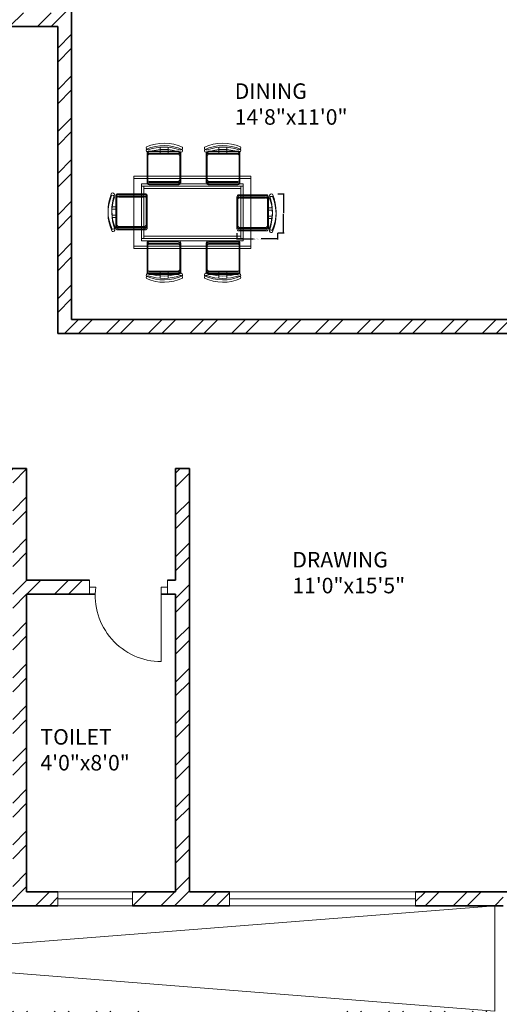
# Model space of a CAD drawing. Units: inches. Extents: x 1885 to 2748, y 783 to 2421.
# Tile 87 of 117: x 2294 to 2449, y 1850 to 2167. Entities that reach past the tile are written whole.
import ezdxf

# ---------------------------------------------------------------- set-up
doc = ezdxf.new("R2010")
doc.units = ezdxf.units.IN
for name, color, linetype, lineweight in [('A-ANNO-DIMS', 2, 'Continuous', 18), ('A-AREA-IDEN', 7, 'Continuous', 18), ('A-DOOR', 31, 'Continuous', 18), ('A-FLOR-OPEN', 8, 'Continuous', 13), ('A-FURN', 8, 'Continuous', 13), ('A-GLAZ', 181, 'Continuous', 18), ('A-WALL', 7, 'Continuous', 35)]:
    doc.layers.add(name, color=color, linetype=linetype, lineweight=lineweight)
doc.layers.add('A-WALL-PATT', color=85, linetype='Continuous', lineweight=13, true_color=0x58ba48)
doc.styles.get("Standard").update_dxf_attribs({"font": 'arial.ttf'})
doc.dimstyles.get("Standard").update_dxf_attribs({"dimtxt": 0.18, "dimasz": 0.18, "dimexe": 0.18, "dimexo": 0.0625, "dimgap": 0.09, "dimtad": 0, "dimtih": 1, "dimtoh": 1, "dimdec": 4, "dimzin": 0, "dimdsep": 46, "dimtxsty": 'Standard', "dimcen": 0.09, "dimadec": 0, "dimazin": 0, "dimtfac": 1, "dimtdec": 4, "dimtofl": 0, "dimtmove": 0, "dimatfit": 3, "dimfxl": 1, "dimtolj": 1, "dimtzin": 0, "dimarcsym": 0})

# ---------------------------------------------------------------- blocks, each defined once
blk = doc.blocks.new('WIN-60')
for p, q in [((0, 60), (4.5, 60)), ((0, 60), (0, 0)), ((4.5, 60), (2.25, 60)), ((2.25, 60), (2.25, 0)), ((4.5, 0), (4.5, 60)), ((2.25, 0), (0, 0)), ((0, 0), (4.5, 0))]:
    blk.add_line(p, q)
blk = doc.blocks.new('WIN-24')
for p, q in [((0, 4.5), (0, 0)), ((0, 4.5), (24, 4.5)), ((24, 2.25), (24, 4.5)), ((24, 4.5), (24, 0)), ((0, 0), (0, 2.25)), ((0, 2.25), (24, 2.25)), ((24, 0), (0, 0))]:
    blk.add_line(p, q)
blk = doc.blocks.new('TABLE-DINING-RECT')
for points in [[(0, 23.42), (37.78, 23.42), (37.78, 0.75), (0, 0.75)], [(0, 23.42), (37.78, 23.42), (37.78, 0.75), (0, 0.75)], [(0, 22.67), (37.78, 22.67), (37.78, 0), (0, 0)], [(0, 22.67), (37.78, 22.67), (37.78, 0), (0, 0)], [(2.51, 20.9), (35.26, 20.9), (35.26, 3.27), (2.51, 3.27)], [(2.51, 20.9), (35.26, 20.9), (35.26, 3.27), (2.51, 3.27)], [(2.51, 20.15), (35.26, 20.15), (35.26, 2.52), (2.51, 2.52)], [(2.51, 20.15), (35.26, 20.15), (35.26, 2.52), (2.51, 2.52)], [(3.27, 20.15), (34.5, 20.15), (34.5, 4.03), (3.27, 4.03)], [(3.27, 20.15), (34.5, 20.15), (34.5, 4.03), (3.27, 4.03)], [(3.27, 19.39), (34.5, 19.39), (34.5, 3.27), (3.27, 3.27)], [(3.27, 19.39), (34.5, 19.39), (34.5, 3.27), (3.27, 3.27)]]:
    blk.add_lwpolyline(points, close=True)
blk = doc.blocks.new('CHAIR-DINING-SIDE-B')
for points in [[(10.8, 3.27, 0.414214), (11.47, 3.94), (11.47, 12.73, 0.414214), (10.8, 13.39), (1.25, 13.39, 0.414214), (0.58, 12.73), (0.58, 3.94, 0.414214), (1.25, 3.27), (10.8, 3.27)], [(10.8, 3.27, 0.414214), (11.47, 3.94), (11.47, 12.73, 0.414214), (10.8, 13.39), (1.25, 13.39, 0.414214), (0.58, 12.73), (0.58, 3.94, 0.414214), (1.25, 3.27), (10.8, 3.27)], [(10.8, 2.52, 0.414214), (11.47, 3.19), (11.47, 11.97, 0.414214), (10.8, 12.64), (1.25, 12.64, 0.414214), (0.58, 11.97), (0.58, 3.19, 0.414214), (1.25, 2.52), (10.8, 2.52)], [(10.8, 2.52, 0.414214), (11.47, 3.19), (11.47, 11.97, 0.414214), (10.8, 12.64), (1.25, 12.64, 0.414214), (0.58, 11.97), (0.58, 3.19, 0.414214), (1.25, 2.52), (10.8, 2.52)], [(4.6, 3.27), (4.6, 2.07, -0.064759)], [(4.6, 3.27), (4.6, 2.07, -0.064759)], [(11.1, 2.86, -0.175809), (0.81, 2.94, 0.578392), (0.03, 2.08, 0.214524), (11.65, 1.93, 0.552014), (11.1, 2.86, -0.065079)], [(11.1, 2.86, -0.175809), (0.81, 2.94, 0.578392), (0.03, 2.08, 0.214524), (11.65, 1.93, 0.552014), (11.1, 2.86, -0.065079)], [(11.1, 2.11, -0.175809), (0.81, 2.18, 0.578392), (0.03, 1.33, 0.214524), (11.65, 1.17, 0.552014), (11.1, 2.11, -0.065079)], [(11.1, 2.1, -0.175809), (0.81, 2.18, 0.578392), (0.03, 1.33, 0.214524), (11.65, 1.17, 0.552014), (11.1, 2.1, -0.065079)], [(4.6, 2.52), (4.6, 1.31, -0.064759)], [(4.6, 2.52), (4.6, 1.31, -0.064759)]]:
    blk.add_lwpolyline(points, format="xyb")
for points in [[(10.8, 3.57), (1.55, 3.57, -0.414214), (0.88, 4.24), (0.88, 12.42, -0.414214), (1.55, 13.09), (10.8, 13.09, -0.512069), (11.17, 12.42), (11.17, 4.24, -0.512069)], [(10.8, 3.57), (1.55, 3.57, -0.414214), (0.88, 4.24), (0.88, 12.42, -0.414214), (1.55, 13.09), (10.8, 13.09, -0.512069), (11.17, 12.42), (11.17, 4.24, -0.512069)], [(10.8, 2.82), (1.55, 2.82, -0.414214), (0.88, 3.49), (0.88, 11.67, -0.414214), (1.55, 12.34), (10.8, 12.34, -0.512069), (11.17, 11.67), (11.17, 3.49, -0.512069)], [(10.8, 2.82), (1.55, 2.82, -0.414214), (0.88, 3.49), (0.88, 11.67, -0.414214), (1.55, 12.34), (10.8, 12.34, -0.512069), (11.17, 11.67), (11.17, 3.49, -0.512069)]]:
    blk.add_lwpolyline(points, format="xyb", close=True)
for points in [[(7.28, 2.04), (7.28, 3.27)], [(7.28, 2.04), (7.28, 3.27)], [(7.28, 1.29), (7.28, 2.52)], [(7.28, 1.29), (7.28, 2.52)]]:
    blk.add_lwpolyline(points)
blk = doc.blocks.new('CHAIR-DINING-END')
for points in [[(10.12, 11.56, 0.414214), (9.45, 12.23), (0.67, 12.23, 0.414214), (0, 11.56), (0, 2.01, 0.414214), (0.67, 1.34), (9.45, 1.34, 0.414214), (10.12, 2.01), (10.12, 11.56)], [(10.12, 11.56, 0.414214), (9.45, 12.23), (0.67, 12.23, 0.414214), (0, 11.56), (0, 2.01, 0.414214), (0.67, 1.34), (9.45, 1.34, 0.414214), (10.12, 2.01), (10.12, 11.56)], [(10.12, 10.81, 0.414214), (9.45, 11.47), (0.67, 11.47, 0.414214), (0, 10.81), (0, 1.25, 0.414214), (0.67, 0.58), (9.45, 0.58, 0.414214), (10.12, 1.25), (10.12, 10.81)], [(10.12, 10.8, 0.414214), (9.45, 11.47), (0.67, 11.47, 0.414214), (0, 10.8), (0, 1.25, 0.414214), (0.67, 0.58), (9.45, 0.58, 0.414214), (10.12, 1.25), (10.12, 10.8)], [(10.53, 11.86, -0.175809), (10.46, 1.57, 0.578392), (11.31, 0.79, 0.214524), (11.47, 12.41, 0.552014), (10.53, 11.86, -0.065079)], [(10.53, 11.86, -0.175809), (10.46, 1.57, 0.578392), (11.31, 0.79, 0.214524), (11.47, 12.41, 0.552014), (10.53, 11.86, -0.065079)], [(10.53, 11.11, -0.175809), (10.46, 0.82, 0.578392), (11.31, 0.04, 0.214524), (11.47, 11.65, 0.552014), (10.53, 11.11, -0.065079)], [(10.53, 11.11, -0.175809), (10.46, 0.82, 0.578392), (11.31, 0.04, 0.214524), (11.47, 11.65, 0.552014), (10.53, 11.11, -0.065079)], [(10.12, 5.36), (11.33, 5.36, -0.064759)], [(10.12, 5.36), (11.33, 5.36, -0.064759)], [(10.12, 4.61), (11.33, 4.61, -0.064759)], [(10.12, 4.61), (11.33, 4.61, -0.064759)]]:
    blk.add_lwpolyline(points, format="xyb")
for points in [[(9.82, 11.56), (9.82, 2.31, -0.414214), (9.15, 1.64), (0.97, 1.64, -0.414214), (0.3, 2.31), (0.3, 11.56, -0.512069), (0.97, 11.93), (9.15, 11.93, -0.512069)], [(9.82, 11.56), (9.82, 2.31, -0.414214), (9.15, 1.64), (0.97, 1.64, -0.414214), (0.3, 2.31), (0.3, 11.56, -0.512069), (0.97, 11.93), (9.15, 11.93, -0.512069)], [(9.82, 10.8), (9.82, 1.55, -0.414214), (9.15, 0.89), (0.97, 0.89, -0.414214), (0.3, 1.55), (0.3, 10.8, -0.512069), (0.97, 11.17), (9.15, 11.17, -0.512069)], [(9.82, 10.8), (9.82, 1.55, -0.414214), (9.15, 0.88), (0.97, 0.88, -0.414214), (0.3, 1.55), (0.3, 10.8, -0.512069), (0.97, 11.17), (9.15, 11.17, -0.512069)]]:
    blk.add_lwpolyline(points, format="xyb", close=True)
for points in [[(11.35, 8.04), (10.12, 8.04)], [(11.35, 8.04), (10.12, 8.04)], [(11.35, 7.28), (10.12, 7.28)], [(11.35, 7.28), (10.12, 7.28)]]:
    blk.add_lwpolyline(points)
blk = doc.blocks.new('*D41')
at = {"layer": 'A-ANNO-DIMS', "color": 0, "lineweight": -2, "transparency": 16777216}
for p, q in [((2364.09, 2098.46), (2364.09, 2096.38)), ((2364.27, 2096.56), (2369.38, 2096.56)), ((2376.99, 2096.56), (2371.88, 2096.56)), ((2377.17, 2098.46), (2377.17, 2096.38))]:
    blk.add_line(p, q, dxfattribs=at)
at = {"layer": 'A-ANNO-DIMS', "color": 0, "transparency": 16777216}
for points in [[(2364.27, 2096.59), (2364.27, 2096.53), (2364.09, 2096.56)], [(2376.99, 2096.59), (2376.99, 2096.53), (2377.17, 2096.56)]]:
    blk.add_solid(points, dxfattribs=at)
at = {"layer": 'Defpoints', "color": 0, "transparency": 16777216}
for p in [(2364.09, 2098.52), (2377.17, 2098.52), (2377.17, 2096.56)]:
    blk.add_point(p, dxfattribs=at)
at = {"layer": 'A-ANNO-DIMS', "color": 0, "transparency": 16777216, "insert": (2370.63, 2096.56), "char_height": 0.18, "attachment_point": 5}
blk.add_mtext('\\A1;END CHAIR 13 TYP.', dxfattribs=at)
blk = doc.blocks.new('*D42')
at = {"layer": 'A-ANNO-DIMS', "color": 0, "lineweight": -2, "transparency": 16777216}
for p, q in [((2377.23, 2111.07), (2379.31, 2111.07)), ((2379.13, 2110.89), (2379.13, 2104.98)), ((2379.13, 2098.7), (2379.13, 2104.61)), ((2377.23, 2098.52), (2379.31, 2098.52))]:
    blk.add_line(p, q, dxfattribs=at)
at = {"layer": 'A-ANNO-DIMS', "color": 0, "transparency": 16777216}
for points in [[(2379.1, 2110.89), (2379.16, 2110.89), (2379.13, 2111.07)], [(2379.1, 2098.7), (2379.16, 2098.7), (2379.13, 2098.52)]]:
    blk.add_solid(points, dxfattribs=at)
at = {"layer": 'Defpoints', "color": 0, "transparency": 16777216}
for p in [(2377.17, 2111.07), (2379.13, 2111.07), (2377.17, 2098.52)]:
    blk.add_point(p, dxfattribs=at)
at = {"layer": 'A-ANNO-DIMS', "color": 0, "transparency": 16777216, "insert": (2379.13, 2104.8), "char_height": 0.18, "attachment_point": 5}
blk.add_mtext('\\A1;13 TYP.', dxfattribs=at)

msp = doc.modelspace()

# ---------------------------------------------------------------- hatches: boundary and pattern name
at = {"layer": 'A-WALL-PATT'}
h = msp.add_hatch(dxfattribs=at)
h.set_pattern_fill('ANSI32', color=256)
h.paths.add_polyline_path([(2007.77, 2318.01), (1980.77, 2318.01), (1980.77, 2281.22), (1985.27, 2281.22), (1985.27, 2313.51), (2007.77, 2313.51), (2007.77, 2315.76)])
h.paths.add_polyline_path([(2094.32, 2318.01), (2067.77, 2318.01), (2067.77, 2313.51), (2094.32, 2313.51), (2094.32, 2315.76)])
h.paths.add_polyline_path([(2131.37, 2315.76), (2131.37, 2318.01), (2131.19, 2318.01), (2112.61, 2318.01), (2112.61, 2313.51), (2117.27, 2313.51), (2117.27, 2255.2), (2121.77, 2255.2), (2121.77, 2313.51), (2131.37, 2313.51)])
h.paths.add_polyline_path([(2190.51, 2318.01), (2155.37, 2318.01), (2155.37, 2313.51), (2169.77, 2313.51), (2169.77, 2229.51), (2121.77, 2229.51), (2121.77, 2233.45), (2119.52, 2233.45), (2117.27, 2233.45), (2117.27, 2201.1), (2121.77, 2201.1), (2121.77, 2225.01), (2169.77, 2225.01), (2169.77, 2165.01), (2306.27, 2165.01), (2306.27, 2066.01), (2310.77, 2066.01), (2344.27, 2066.01), (2486.27, 2066.01), (2486.27, 1886.01), (2483.02, 1886.01), (2483.02, 1881.51), (2486.27, 1881.51), (2486.27, 1880.68), (2490.77, 1880.68), (2490.77, 2070.51), (2344.27, 2070.51), (2310.77, 2070.51), (2310.77, 2165.01), (2310.77, 2173.64), (2308.52, 2173.64), (2306.27, 2173.64), (2306.27, 2169.51), (2174.27, 2169.51), (2174.27, 2313.51), (2190.51, 2313.51), (2190.51, 2315.76)])
h.paths.add_polyline_path([(1985.27, 2221.22), (1980.77, 2221.22), (1980.77, 2165.01), (1992.77, 2165.01), (1992.77, 2141.93), (1997.27, 2141.93), (1997.27, 2165.01), (2117.27, 2165.01), (2117.27, 2163.13), (2121.77, 2163.13), (2121.77, 2172.73), (2119.52, 2172.73), (2117.27, 2172.73), (2117.27, 2169.51), (1985.27, 2169.51)])
h.paths.add_polyline_path([(1997.27, 2105.93), (1992.77, 2105.93), (1992.77, 2070.51), (2016.77, 2070.51), (2016.77, 2059.12), (2019.02, 2059.12), (2021.27, 2059.12), (2021.27, 2070.51), (2117.27, 2070.51), (2117.27, 2022.51), (2114.42, 2022.51), (2114.42, 2018.01), (2123.63, 2018.01), (2123.63, 2020.26), (2123.63, 2022.51), (2121.77, 2022.51), (2121.77, 2142.59), (2119.52, 2142.59), (2117.27, 2142.59), (2117.27, 2075.01), (1997.27, 2075.01)])
h.paths.add_polyline_path([(2092.03, 2020.26), (2092.03, 2022.51), (2021.27, 2022.51), (2021.27, 2035.12), (2016.77, 2035.12), (2016.77, 2018.01), (2016.77, 1978.78), (2021.27, 1978.78), (2021.27, 2018.01), (2092.03, 2018.01)])
h.paths.add_polyline_path([(2260.94, 2022.51), (2153.1, 2022.51), (2153.1, 2020.26), (2153.1, 2018.01), (2155.27, 2018.01), (2155.27, 1886.01), (2107.63, 1886.01), (2107.63, 1881.51), (2182.91, 1881.51), (2182.91, 1883.76), (2182.91, 1886.01), (2159.77, 1886.01), (2159.77, 2018.01), (2260.94, 2018.01), (2260.94, 2020.26)])
h.paths.add_polyline_path([(2047.63, 1883.76), (2047.63, 1886.01), (2021.27, 1886.01), (2021.27, 1918.78), (2019.02, 1918.78), (2016.77, 1918.78), (2016.77, 1881.51), (2047.63, 1881.51)])
h.paths.add_polyline_path([(2306.36, 1883.76), (2306.36, 1886.01), (2296.27, 1886.01), (2296.27, 1982.01), (2316.54, 1982.01), (2316.54, 1984.26), (2316.54, 1986.51), (2296.27, 1986.51), (2296.27, 2022.51), (2289.28, 2022.51), (2289.28, 2018.01), (2291.77, 2018.01), (2291.77, 1886.01), (2242.91, 1886.01), (2242.91, 1881.51), (2306.36, 1881.51)], flags=17)
h.paths.add_polyline_path([(1985.27, 1843.01), (2021.6, 1843.01), (2021.53, 1845.44), (2021.48, 1847.51), (1980.77, 1847.51), (1980.77, 1809.45), (1985.27, 1809.45)])
h.paths.add_polyline_path([(2131.48, 1845.26), (2131.48, 1847.51), (2081.53, 1847.51), (2081.53, 1843.01), (2117.27, 1843.01), (2117.27, 1784.15), (2119.52, 1784.15), (2121.77, 1784.15), (2121.77, 1843.01), (2131.48, 1843.01)])
h.paths.add_polyline_path([(2203.89, 1847.51), (2155.48, 1847.51), (2155.48, 1843.01), (2169.77, 1843.01), (2169.77, 1759.01), (2121.77, 1759.01), (2121.77, 1761.46), (2117.27, 1761.46), (2117.27, 1730.43), (2121.77, 1730.43), (2121.77, 1754.51), (2177.42, 1754.51), (2177.42, 1756.76), (2177.42, 1759.01), (2174.27, 1759.01), (2174.27, 1843.01), (2203.89, 1843.01)])
h.paths.add_polyline_path([(2335.55, 1845.26), (2335.55, 1847.51), (2239.89, 1847.51), (2239.89, 1843.01), (2306.27, 1843.01), (2306.27, 1759.01), (2199.49, 1759.01), (2199.49, 1754.51), (2310.77, 1754.51), (2310.77, 1843.01), (2335.55, 1843.01)])
h.paths.add_polyline_path([(2348.77, 2022.51), (2344.27, 2022.51), (2344.27, 1986.51), (2341.68, 1986.51), (2341.68, 1982.01), (2344.27, 1982.01), (2344.27, 1886.01), (2330.36, 1886.01), (2330.36, 1881.51), (2361.63, 1881.51), (2361.63, 1883.76), (2361.63, 1886.01), (2348.77, 1886.01)], flags=17)
h.paths.add_polyline_path([(2283.25, 2315.76), (2283.25, 2318.01), (2238.51, 2318.01), (2238.51, 2313.51), (2283.25, 2313.51)], flags=17)
h.paths.add_polyline_path([(2363.27, 2348.01), (2388.68, 2348.01), (2388.68, 2350.26), (2388.68, 2352.51), (2358.77, 2352.51), (2358.77, 2348.01), (2358.77, 2318.01), (2344.48, 2318.01), (2344.48, 2313.51), (2358.77, 2313.51), (2358.77, 2229.51), (2310.77, 2229.51), (2310.77, 2231.95), (2306.27, 2231.95), (2306.27, 2205.61), (2310.77, 2205.61), (2310.77, 2225.01), (2358.77, 2225.01), (2358.77, 2211.51), (2452.33, 2211.51), (2452.33, 2213.76), (2452.33, 2216.01), (2363.27, 2216.01), (2363.27, 2318.01)])
h.paths.add_polyline_path([(2310.77, 2313.51), (2320.48, 2313.51), (2320.48, 2315.76), (2320.48, 2318.01), (2302.73, 2318.01), (2302.73, 2313.51), (2306.27, 2313.51), (2306.27, 2251.08), (2310.77, 2251.08)], flags=17)
h.paths.add_polyline_path([(2490.77, 2352.51), (2486.27, 2352.51), (2448.68, 2352.51), (2448.68, 2348.01), (2486.27, 2348.01), (2486.27, 2318.01), (2486.27, 2216.01), (2481.78, 2216.01), (2481.78, 2211.51), (2486.27, 2211.51), (2486.27, 2165.01), (2493.29, 2165.01), (2493.29, 2167.26), (2493.29, 2169.51), (2490.77, 2169.51), (2490.77, 2313.51), (2494.43, 2313.51), (2494.43, 2318.01), (2490.77, 2318.01)])
h.paths.add_polyline_path([(2534.65, 2318.01), (2515.69, 2318.01), (2515.69, 2313.51), (2534.65, 2313.51), (2534.65, 2315.76)])
h.paths.add_polyline_path([(2618.27, 2318.01), (2594.65, 2318.01), (2594.65, 2313.51), (2613.77, 2313.51), (2613.77, 2281.71), (2618.27, 2281.71)])
h.paths.add_polyline_path([(2618.27, 2221.71), (2613.77, 2221.71), (2613.77, 2169.51), (2554.02, 2169.51), (2554.02, 2165.01), (2613.77, 2165.01), (2613.77, 2152.88), (2618.27, 2152.88)])
h.paths.add_polyline_path([(2618.27, 2128.88), (2616.02, 2128.88), (2613.77, 2128.88), (2613.77, 2117.01), (2529.77, 2117.01), (2529.77, 2165.01), (2532.85, 2165.01), (2532.85, 2169.51), (2522.87, 2169.51), (2522.87, 2165.01), (2525.27, 2165.01), (2525.27, 2117.01), (2525.27, 2112.51), (2525.27, 2108.58), (2529.77, 2108.58), (2529.77, 2112.51), (2613.77, 2112.51), (2613.77, 2080.19), (2618.27, 2080.19)])
h.paths.add_polyline_path([(2618.27, 2044.19), (2616.02, 2044.19), (2613.77, 2044.19), (2613.77, 2015.51), (2529.77, 2015.51), (2529.77, 2088.58), (2527.52, 2088.58), (2525.27, 2088.58), (2525.27, 2011.01), (2613.77, 2011.01), (2613.77, 1956.75), (2618.27, 1956.75)])
h.paths.add_polyline_path([(2618.27, 1881.51), (2618.27, 1896.75), (2613.77, 1896.75), (2613.77, 1881.51), (2613.77, 1847.51), (2592.71, 1847.51), (2592.71, 1843.01), (2613.77, 1843.01), (2613.77, 1765.01), (2613.77, 1760.51), (2609.62, 1760.51), (2609.62, 1756.01), (2613.77, 1756.01), (2613.77, 1660.01), (2608.54, 1660.01), (2608.54, 1655.51), (2613.77, 1655.51), (2613.77, 1508.16), (2618.27, 1508.16)])
h.paths.add_polyline_path([(2565.77, 1843.01), (2569, 1843.01), (2569, 1847.51), (2490.77, 1847.51), (2490.77, 1849.7), (2488.52, 1849.7), (2486.27, 1849.7), (2486.27, 1847.51), (2477.27, 1847.51), (2477.27, 1838.51), (2477.27, 1821.49), (2486.27, 1821.49), (2486.27, 1838.51), (2561.27, 1838.51), (2561.27, 1765.01), (2486.27, 1765.01), (2486.27, 1786.16), (2477.27, 1786.16), (2477.27, 1765.01), (2477.27, 1756.01), (2486.27, 1756.01), (2565.77, 1756.01), (2585.62, 1756.01), (2585.62, 1758.26), (2585.62, 1760.51), (2565.77, 1760.51), (2565.77, 1765.01)])
h.paths.add_polyline_path([(2486.27, 1651.01), (2561.27, 1651.01), (2561.27, 1567.01), (2486.27, 1567.01), (2486.27, 1591.32), (2477.27, 1591.32), (2477.27, 1567.01), (2477.27, 1558.01), (2477.27, 1555.44), (2481.77, 1555.44), (2481.77, 1558.01), (2568.65, 1558.01), (2568.65, 1560.26), (2568.65, 1562.51), (2565.77, 1562.51), (2565.77, 1655.51), (2584.54, 1655.51), (2584.54, 1657.76), (2584.54, 1660.01), (2565.77, 1660.01), (2486.27, 1660.01), (2477.27, 1660.01), (2477.27, 1651.01), (2477.27, 1632.99), (2486.27, 1632.99)])
h.paths.add_polyline_path([(2449.97, 1883.76), (2449.97, 1886.01), (2421.63, 1886.01), (2421.63, 1881.51), (2449.97, 1881.51)], flags=17)
h.paths.add_polyline_path([(2447.27, 1847.51), (2395.55, 1847.51), (2395.55, 1843.01), (2442.77, 1843.01), (2442.77, 1809.27), (2447.27, 1809.27)])
h.paths.add_polyline_path([(1985.27, 1749.45), (1980.77, 1749.45), (1980.77, 1694.5), (1985.27, 1694.5), (1985.27, 1694.51), (1986.9, 1694.51), (1986.9, 1697.78), (1986.9, 1699.01), (1985.27, 1699.01)])
h.paths.add_polyline_path([(2152.77, 1699.01), (2121.77, 1699.01), (2121.77, 1703.67), (2119.52, 1703.67), (2117.27, 1703.67), (2117.27, 1699.01), (2009.22, 1699.01), (2009.22, 1694.51), (2148.27, 1694.51), (2148.27, 1692.63), (2152.77, 1692.63)])
h.paths.add_polyline_path([(2016.27, 1694.51), (2011.77, 1694.51), (2011.77, 1558.01), (2040.81, 1558.01), (2040.81, 1560.26), (2040.81, 1562.51), (2016.27, 1562.51)])
h.paths.add_polyline_path([(2152.77, 1663.02), (2150.52, 1663.02), (2148.27, 1663.02), (2148.27, 1562.51), (2100.81, 1562.51), (2100.81, 1558.01), (2165.12, 1558.01), (2165.12, 1560.26), (2165.12, 1562.51), (2152.77, 1562.51), (2152.77, 1610.51), (2224.77, 1610.51), (2224.77, 1607.99), (2229.27, 1607.99), (2229.27, 1615.01), (2152.77, 1615.01)])
h.paths.add_polyline_path([(2238.61, 1560.26), (2238.61, 1562.51), (2229.27, 1562.51), (2229.27, 1588.76), (2227.02, 1588.76), (2224.77, 1588.77), (2224.77, 1562.51), (2189.12, 1562.51), (2189.12, 1558.01), (2238.61, 1558.01)])
h.paths.add_polyline_path([(2336.02, 1560.26), (2336.02, 1562.51), (2310.77, 1562.51), (2310.77, 1656.35), (2308.52, 1656.35), (2306.27, 1656.35), (2306.27, 1562.51), (2286.61, 1562.51), (2286.61, 1558.01), (2336.02, 1558.01)])
h.paths.add_polyline_path([(2447.27, 1690.97), (2445.02, 1690.97), (2442.77, 1690.97), (2442.77, 1687.01), (2306.27, 1687.01), (2306.27, 1680.75), (2310.77, 1680.75), (2310.77, 1682.51), (2442.77, 1682.51), (2442.77, 1562.51), (2396.02, 1562.51), (2396.02, 1558.01), (2447.27, 1558.01)])
h.paths.add_polyline_path([(2447.27, 1749.27), (2445.02, 1749.27), (2442.77, 1749.27), (2442.77, 1717.23), (2447.27, 1717.23)])
h.paths.add_polyline_path([(2044.67, 1521.76), (2044.67, 1524.01), (2007.27, 1524.01), (2007.27, 1503.49), (2009.52, 1503.49), (2011.77, 1503.49), (2011.77, 1519.51), (2044.67, 1519.51)])
h.paths.add_polyline_path([(2177.97, 1521.76), (2177.97, 1524.01), (2104.67, 1524.01), (2104.67, 1519.51), (2145.77, 1519.51), (2145.77, 1387.51), (2143.37, 1387.51), (2143.37, 1383.01), (2251.59, 1383.01), (2251.59, 1385.26), (2251.59, 1387.51), (2150.27, 1387.51), (2150.27, 1519.51), (2177.97, 1519.51)])
h.paths.add_polyline_path([(2298.7, 1524.01), (2237.97, 1524.01), (2237.97, 1519.51), (2282.27, 1519.51), (2282.27, 1387.51), (2279.68, 1387.51), (2279.68, 1383.01), (2286.77, 1383.01), (2286.77, 1419.01), (2312.45, 1419.01), (2312.45, 1421.26), (2312.45, 1423.51), (2286.77, 1423.51), (2286.77, 1519.51), (2298.7, 1519.51), (2298.7, 1521.72)], flags=17)
h.paths.add_polyline_path([(2361.9, 1521.76), (2361.9, 1524.01), (2322.7, 1524.01), (2322.7, 1519.51), (2334.77, 1519.51), (2334.77, 1423.51), (2331.93, 1423.51), (2331.93, 1419.01), (2334.77, 1419.01), (2334.77, 1387.51), (2334.77, 1383.23), (2339.27, 1383.23), (2339.27, 1387.51), (2339.27, 1519.51), (2361.9, 1519.51)], flags=17)
h.paths.add_polyline_path([(2447.27, 1521.76), (2447.27, 1524.01), (2421.9, 1524.01), (2421.9, 1519.51), (2447.27, 1519.51)], flags=17)
h.paths.add_polyline_path([(2481.77, 1529.6), (2479.52, 1529.6), (2477.27, 1529.6), (2477.27, 1524.01), (2474.49, 1524.01), (2474.49, 1519.51), (2477.27, 1519.51), (2477.27, 1334.51), (2296.77, 1334.51), (2296.77, 1240.51), (2160.27, 1240.51), (2160.27, 1180.51), (2112.27, 1180.51), (2112.27, 1207.69), (2110.02, 1207.69), (2107.77, 1207.69), (2107.77, 1171.61), (2112.27, 1171.61), (2112.27, 1176.01), (2160.27, 1176.01), (2160.27, 1092.01), (2144.22, 1092.01), (2144.22, 1087.51), (2189.5, 1087.51), (2189.5, 1089.76), (2189.5, 1092.01), (2164.77, 1092.01), (2164.77, 1236.01), (2296.77, 1236.01), (2296.77, 1231.91), (2301.27, 1231.91), (2301.27, 1330.01), (2481.77, 1330.01), (2481.77, 1387.51)])
h.paths.add_polyline_path([(2618.27, 1448.16), (2613.77, 1448.16), (2613.77, 1382.51), (2529.77, 1382.51), (2525.27, 1382.51), (2525.27, 1307.06), (2529.77, 1307.06), (2529.77, 1378.01), (2613.77, 1378.01), (2613.77, 1354.99), (2618.27, 1354.99)])
h.paths.add_polyline_path([(2618.27, 1318.99), (2613.77, 1318.99), (2613.77, 1281.01), (2529.77, 1281.01), (2529.77, 1283.79), (2527.52, 1283.79), (2525.27, 1283.79), (2525.27, 1228.51), (2516.79, 1228.51), (2516.79, 1224.01), (2533.48, 1224.01), (2533.48, 1226.26), (2533.48, 1228.51), (2529.77, 1228.51), (2529.77, 1276.51), (2613.77, 1276.51), (2613.77, 1266.02), (2618.27, 1266.02)])
h.paths.add_polyline_path([(2618.27, 1134.96), (2613.77, 1134.96), (2613.77, 1092.01), (2594.54, 1092.01), (2594.54, 1087.51), (2618.27, 1087.51)])
h.paths.add_polyline_path([(2534.54, 1092.01), (2509.77, 1092.01), (2509.77, 1087.51), (2534.54, 1087.51), (2534.54, 1089.76)])
h.paths.add_polyline_path([(2481.27, 1224.01), (2484.12, 1224.01), (2484.12, 1226.26), (2484.12, 1228.51), (2476.77, 1228.51), (2476.77, 1198.51), (2471.61, 1198.51), (2471.61, 1194.01), (2476.77, 1194.01), (2476.77, 1062.01), (2436.89, 1062.01), (2436.89, 1057.51), (2476.77, 1057.51), (2481.27, 1057.51), (2481.27, 1062.01), (2481.27, 1087.51), (2485.35, 1087.51), (2485.35, 1089.76), (2485.35, 1092.01), (2481.27, 1092.01), (2481.27, 1117.51)])
h.paths.add_polyline_path([(2439.9, 1198.51), (2349.27, 1198.51), (2349.27, 1194.01), (2349.27, 1180.51), (2301.27, 1180.51), (2301.27, 1201.9), (2299.02, 1201.9), (2296.77, 1201.9), (2296.77, 1172.34), (2299.02, 1172.34), (2301.27, 1172.34), (2301.27, 1176.01), (2349.27, 1176.01), (2349.27, 1092.01), (2334.45, 1092.01), (2334.45, 1087.51), (2349.27, 1087.51), (2349.27, 1057.51), (2353.77, 1057.51), (2376.89, 1057.51), (2376.89, 1059.76), (2376.89, 1062.01), (2353.77, 1062.01), (2353.77, 1087.51), (2353.77, 1180.51), (2353.77, 1194.01), (2439.9, 1194.01), (2439.9, 1196.26)])
h.paths.add_polyline_path([(2270.6, 1089.76), (2270.6, 1092.01), (2249.5, 1092.01), (2249.5, 1087.51), (2270.6, 1087.51)], flags=17)
h.paths.add_polyline_path([(2310.45, 1092.01), (2301.27, 1092.01), (2301.27, 1153.29), (2296.77, 1153.29), (2296.77, 1092.01), (2293.79, 1092.01), (2293.79, 1087.51), (2310.45, 1087.51), (2310.45, 1089.76)], flags=17)
h.paths.add_polyline_path([(2112.27, 1150.33), (2110.02, 1150.33), (2107.77, 1150.33), (2107.77, 1092.01), (2104.47, 1092.01), (2104.47, 1087.51), (2120.22, 1087.51), (2120.22, 1089.76), (2120.22, 1092.01), (2112.27, 1092.01)])
h.paths.add_polyline_path([(2082.17, 1092.01), (2058.14, 1092.01), (2058.14, 1087.51), (2082.17, 1087.51), (2082.17, 1089.76)])
h.paths.add_polyline_path([(1975.77, 1145.64), (1971.27, 1145.64), (1971.27, 1087.51), (1980.77, 1087.51), (1998.14, 1087.51), (1998.14, 1089.76), (1998.14, 1092.01), (1985.27, 1092.01), (1975.77, 1092.01)])
h.paths.add_polyline_path([(2112.27, 1244.38), (2110.02, 1244.38), (2107.77, 1244.38), (2107.77, 1240.51), (1992.27, 1240.51), (1992.27, 1271.01), (1987.77, 1271.01), (1987.77, 1240.51), (1980.77, 1240.51), (1975.77, 1240.51), (1971.27, 1240.51), (1971.27, 1205.64), (1975.77, 1205.64), (1975.77, 1236.01), (2107.77, 1236.01), (2107.77, 1233.44), (2112.27, 1233.44), (2112.27, 1236.01)])
h.paths.add_polyline_path([(2112.27, 1383.01), (2114.78, 1383.01), (2114.78, 1385.26), (2114.78, 1387.51), (2102.48, 1387.51), (2102.48, 1383.01), (2107.77, 1383.01), (2107.77, 1335.01), (2011.77, 1335.01), (2011.77, 1349.94), (2007.27, 1349.94), (2007.27, 1335.01), (1987.77, 1335.01), (1987.77, 1330.51), (1987.77, 1307.01), (1992.27, 1307.01), (1992.27, 1330.51), (2007.27, 1330.51), (2107.77, 1330.51), (2107.77, 1264.71), (2112.27, 1264.71)])
h.paths.add_polyline_path([(2077.86, 1387.51), (2011.77, 1387.51), (2011.77, 1390.04), (2009.52, 1390.04), (2007.27, 1390.04), (2007.27, 1373.94), (2011.77, 1373.94), (2011.77, 1383.01), (2077.86, 1383.01)])
h.paths.add_polyline_path([(2011.77, 1443.49), (2007.27, 1443.49), (2007.27, 1410.25), (2011.77, 1410.25)])

# ---------------------------------------------------------------- linework, layer by layer
at = {"layer": 'A-DOOR'}
for p, q in [((2316.54, 1986.51), (2316.54, 1982.01)), ((2341.68, 1986.51), (2341.68, 1982.01)), ((2316.54, 1982.01), (2316.54, 1984.26)), ((2316.54, 1984.26), (2318.54, 1984.26)), ((2341.68, 1984.26), (2339.68, 1984.26)), ((2339.68, 1984.26), (2339.68, 1960.26)), ((2341.68, 1982.01), (2341.68, 1984.26))]:
    msp.add_line(p, q, dxfattribs=at)
msp.add_arc((2339.68, 1981.57), 21.32, 172.765, 270, dxfattribs=at)
at = {"layer": 'A-FLOR-OPEN'}
for p, q in [((2016.77, 1847.51), (2447.27, 1881.51)), ((2447.27, 1847.51), (2016.77, 1881.51)), ((2447.27, 1847.51), (2447.27, 1881.51))]:
    msp.add_line(p, q, dxfattribs=at)
at = {"layer": 'A-FURN'}
for points in [[(2335.45, 2125.31, -0.175809), (2345.74, 2125.23, 0.578392), (2346.52, 2126.09, 0.214524), (2334.9, 2126.24, 0.552014), (2335.45, 2125.31, -0.065079)], [(2335.45, 2125.31, -0.175809), (2345.74, 2125.23, 0.578392), (2346.52, 2126.09, 0.214524), (2334.9, 2126.24, 0.552014), (2335.45, 2125.31, -0.065079)], [(2335.45, 2124.55, -0.175809), (2345.74, 2124.47, 0.578392), (2346.52, 2125.33, 0.214524), (2334.9, 2125.49, 0.552014), (2335.45, 2124.55, -0.065079)], [(2335.45, 2124.55, -0.175809), (2345.74, 2124.47, 0.578392), (2346.52, 2125.33, 0.214524), (2334.9, 2125.49, 0.552014), (2335.45, 2124.55, -0.065079)], [(2345.3, 2124.89), (2335.75, 2124.89, 0.414214), (2335.08, 2124.23), (2335.08, 2115.44, 0.414214), (2335.75, 2114.77), (2345.3, 2114.77, 0.414214), (2345.97, 2115.44), (2345.97, 2124.23, 0.414214), (2345.3, 2124.89)], [(2345.3, 2124.89), (2335.75, 2124.89, 0.414214), (2335.08, 2124.23), (2335.08, 2115.44, 0.414214), (2335.75, 2114.77), (2345.3, 2114.77, 0.414214), (2345.97, 2115.44), (2345.97, 2124.23, 0.414214), (2345.3, 2124.89)], [(2341.95, 2124.89), (2341.95, 2126.1, -0.064759)], [(2341.95, 2124.89), (2341.95, 2126.1, -0.064759)], [(2341.95, 2124.14), (2341.95, 2125.35, -0.064759)], [(2341.95, 2124.14), (2341.95, 2125.35, -0.064759)], [(2354.4, 2125.23, -0.578392), (2353.62, 2126.09, -0.214524), (2365.24, 2126.24, -0.552014), (2364.69, 2125.31, 0.175809), (2354.4, 2125.23)], [(2354.4, 2125.23, -0.578392), (2353.62, 2126.09, -0.214524), (2365.24, 2126.24, -0.552014), (2364.69, 2125.31, 0.175809), (2354.4, 2125.23)], [(2354.4, 2124.47, -0.578392), (2353.62, 2125.33, -0.214524), (2365.24, 2125.49, -0.552014), (2364.69, 2124.55, 0.175809), (2354.4, 2124.47)], [(2354.4, 2124.47, -0.578392), (2353.62, 2125.33, -0.214524), (2365.24, 2125.49, -0.552014), (2364.69, 2124.55, 0.175809), (2354.4, 2124.47)], [(2364.39, 2124.89, -0.414214), (2365.06, 2124.23), (2365.06, 2115.44, -0.414214), (2364.39, 2114.77), (2354.84, 2114.77, -0.414214), (2354.17, 2115.44), (2354.17, 2124.23, -0.414214), (2354.84, 2124.89), (2364.39, 2124.89)], [(2364.39, 2124.89, -0.414214), (2365.06, 2124.23), (2365.06, 2115.44, -0.414214), (2364.39, 2114.77), (2354.84, 2114.77, -0.414214), (2354.17, 2115.44), (2354.17, 2124.23, -0.414214), (2354.84, 2124.89), (2364.39, 2124.89)], [(2358.19, 2124.89), (2358.19, 2126.1, 0.064759)], [(2358.19, 2124.89), (2358.19, 2126.1, 0.064759)], [(2358.19, 2124.14), (2358.19, 2125.35, 0.064759)], [(2358.19, 2124.14), (2358.19, 2125.35, 0.064759)], [(2345.3, 2124.14), (2335.75, 2124.14, 0.414214), (2335.08, 2123.47), (2335.08, 2114.69, 0.414214), (2335.75, 2114.02), (2345.3, 2114.02, 0.414214), (2345.97, 2114.69), (2345.97, 2123.47, 0.414214), (2345.3, 2124.14)], [(2345.3, 2124.14), (2335.75, 2124.14, 0.414214), (2335.08, 2123.47), (2335.08, 2114.69, 0.414214), (2335.75, 2114.02), (2345.3, 2114.02, 0.414214), (2345.97, 2114.69), (2345.97, 2123.47, 0.414214), (2345.3, 2124.14)], [(2364.39, 2124.14, -0.414214), (2365.06, 2123.47), (2365.06, 2114.69, -0.414214), (2364.39, 2114.02), (2354.84, 2114.02, -0.414214), (2354.17, 2114.69), (2354.17, 2123.47, -0.414214), (2354.84, 2124.14), (2364.39, 2124.14)], [(2364.39, 2124.14, -0.414214), (2365.06, 2123.47), (2365.06, 2114.69, -0.414214), (2364.39, 2114.02), (2354.84, 2114.02, -0.414214), (2354.17, 2114.69), (2354.17, 2123.47, -0.414214), (2354.84, 2124.14), (2364.39, 2124.14)], [(2324.68, 2100.46, -0.578392), (2323.83, 2099.68, -0.214524), (2323.67, 2111.29, -0.552014), (2324.6, 2110.75, 0.175809), (2324.68, 2100.46)], [(2324.68, 2100.46, -0.578392), (2323.83, 2099.68, -0.214524), (2323.67, 2111.29, -0.552014), (2324.6, 2110.75, 0.175809), (2324.68, 2100.46)], [(2324.68, 2099.7, -0.578392), (2323.83, 2098.92, -0.214524), (2323.67, 2110.54, -0.552014), (2324.6, 2109.99, 0.175809), (2324.68, 2099.7)], [(2324.68, 2099.7, -0.578392), (2323.83, 2098.92, -0.214524), (2323.67, 2110.54, -0.552014), (2324.6, 2109.99, 0.175809), (2324.68, 2099.7)], [(2325.02, 2110.45, -0.414214), (2325.69, 2111.12), (2334.47, 2111.12, -0.414214), (2335.14, 2110.45), (2335.14, 2100.9, -0.414214), (2334.47, 2100.23), (2325.69, 2100.23, -0.414214), (2325.02, 2100.9), (2325.02, 2110.45)], [(2325.02, 2110.45, -0.414214), (2325.69, 2111.12), (2334.47, 2111.12, -0.414214), (2335.14, 2110.45), (2335.14, 2100.89, -0.414214), (2334.47, 2100.23), (2325.69, 2100.23, -0.414214), (2325.02, 2100.89), (2325.02, 2110.45)], [(2325.02, 2109.69, -0.414214), (2325.69, 2110.36), (2334.47, 2110.36, -0.414214), (2335.14, 2109.69), (2335.14, 2100.14, -0.414214), (2334.47, 2099.47), (2325.69, 2099.47, -0.414214), (2325.02, 2100.14), (2325.02, 2109.69)], [(2325.02, 2109.69, -0.414214), (2325.69, 2110.36), (2334.47, 2110.36, -0.414214), (2335.14, 2109.69), (2335.14, 2100.14, -0.414214), (2334.47, 2099.47), (2325.69, 2099.47, -0.414214), (2325.02, 2100.14), (2325.02, 2109.69)], [(2325.02, 2104.25), (2323.81, 2104.25, 0.064759)], [(2325.02, 2104.25), (2323.81, 2104.25, 0.064759)], [(2325.02, 2103.49), (2323.81, 2103.49, 0.064759)], [(2325.02, 2103.49), (2323.81, 2103.49, 0.064759)], [(2345.3, 2085.85), (2335.75, 2085.85, -0.414214), (2335.08, 2086.52), (2335.08, 2095.3, -0.414214), (2335.75, 2095.97), (2345.3, 2095.97, -0.414214), (2345.97, 2095.3), (2345.97, 2086.52, -0.414214), (2345.3, 2085.85)], [(2345.3, 2085.85), (2335.75, 2085.85, -0.414214), (2335.08, 2086.52), (2335.08, 2095.3, -0.414214), (2335.75, 2095.97), (2345.3, 2095.97, -0.414214), (2345.97, 2095.3), (2345.97, 2086.52, -0.414214), (2345.3, 2085.85)], [(2345.3, 2085.09), (2335.75, 2085.09, -0.414214), (2335.08, 2085.76), (2335.08, 2094.55, -0.414214), (2335.75, 2095.21), (2345.3, 2095.21, -0.414214), (2345.97, 2094.55), (2345.97, 2085.76, -0.414214), (2345.3, 2085.09)], [(2345.3, 2085.09), (2335.75, 2085.09, -0.414214), (2335.08, 2085.76), (2335.08, 2094.54, -0.414214), (2335.75, 2095.21), (2345.3, 2095.21, -0.414214), (2345.97, 2094.54), (2345.97, 2085.76, -0.414214), (2345.3, 2085.09)], [(2345.74, 2085.51, -0.578392), (2346.52, 2084.66, -0.214524), (2334.9, 2084.5, -0.552014), (2335.45, 2085.44, 0.175809), (2345.74, 2085.51)], [(2345.74, 2085.51, -0.578392), (2346.52, 2084.66, -0.214524), (2334.9, 2084.5, -0.552014), (2335.45, 2085.44, 0.175809), (2345.74, 2085.51)], [(2345.74, 2084.76, -0.578392), (2346.52, 2083.9, -0.214524), (2334.9, 2083.74, -0.552014), (2335.45, 2084.68, 0.175809), (2345.74, 2084.76)], [(2345.74, 2084.76, -0.578392), (2346.52, 2083.9, -0.214524), (2334.9, 2083.74, -0.552014), (2335.45, 2084.68, 0.175809), (2345.74, 2084.76)], [(2341.95, 2085.85), (2341.95, 2084.64, 0.064759)], [(2341.95, 2085.85), (2341.95, 2084.64, 0.064759)], [(2341.95, 2085.09), (2341.95, 2083.88, 0.064759)], [(2341.95, 2085.09), (2341.95, 2083.88, 0.064759)]]:
    msp.add_lwpolyline(points, format="xyb", dxfattribs=at)
for points in [[(2335.75, 2124.59), (2345, 2124.59, -0.414214), (2345.67, 2123.92), (2345.67, 2115.74, -0.414214), (2345, 2115.08), (2335.75, 2115.08, -0.512069), (2335.38, 2115.74), (2335.38, 2123.92, -0.512069)], [(2335.75, 2124.59), (2345, 2124.59, -0.414214), (2345.67, 2123.92), (2345.67, 2115.74, -0.414214), (2345, 2115.07), (2335.75, 2115.07, -0.512069), (2335.38, 2115.74), (2335.38, 2123.92, -0.512069)], [(2364.39, 2124.59), (2355.14, 2124.59, 0.414214), (2354.47, 2123.92), (2354.47, 2115.74, 0.414214), (2355.14, 2115.08), (2364.39, 2115.08, 0.512069), (2364.76, 2115.74), (2364.76, 2123.92, 0.512069)], [(2364.39, 2124.59), (2355.14, 2124.59, 0.414214), (2354.47, 2123.92), (2354.47, 2115.74, 0.414214), (2355.14, 2115.07), (2364.39, 2115.07, 0.512069), (2364.76, 2115.74), (2364.76, 2123.92, 0.512069)], [(2335.75, 2123.84), (2345, 2123.84, -0.414214), (2345.67, 2123.17), (2345.67, 2114.99, -0.414214), (2345, 2114.32), (2335.75, 2114.32, -0.512069), (2335.38, 2114.99), (2335.38, 2123.17, -0.512069)], [(2335.75, 2123.84), (2345, 2123.84, -0.414214), (2345.67, 2123.17), (2345.67, 2114.99, -0.414214), (2345, 2114.32), (2335.75, 2114.32, -0.512069), (2335.38, 2114.99), (2335.38, 2123.17, -0.512069)], [(2364.39, 2123.84), (2355.14, 2123.84, 0.414214), (2354.47, 2123.17), (2354.47, 2114.99, 0.414214), (2355.14, 2114.32), (2364.39, 2114.32, 0.512069), (2364.76, 2114.99), (2364.76, 2123.17, 0.512069)], [(2364.39, 2123.84), (2355.14, 2123.84, 0.414214), (2354.47, 2123.17), (2354.47, 2114.99, 0.414214), (2355.14, 2114.32), (2364.39, 2114.32, 0.512069), (2364.76, 2114.99), (2364.76, 2123.17, 0.512069)], [(2325.32, 2110.44), (2325.32, 2101.2, 0.414214), (2325.99, 2100.53), (2334.17, 2100.53, 0.414214), (2334.84, 2101.2), (2334.84, 2110.44, 0.512069), (2334.17, 2110.82), (2325.99, 2110.82, 0.512069)], [(2325.32, 2110.44), (2325.32, 2101.2, 0.414214), (2325.99, 2100.53), (2334.17, 2100.53, 0.414214), (2334.84, 2101.2), (2334.84, 2110.44, 0.512069), (2334.17, 2110.81), (2325.99, 2110.81, 0.512069)], [(2325.32, 2109.69), (2325.32, 2100.44, 0.414214), (2325.99, 2099.77), (2334.17, 2099.77, 0.414214), (2334.84, 2100.44), (2334.84, 2109.69, 0.512069), (2334.17, 2110.06), (2325.99, 2110.06, 0.512069)], [(2325.32, 2109.69), (2325.32, 2100.44, 0.414214), (2325.99, 2099.77), (2334.17, 2099.77, 0.414214), (2334.84, 2100.44), (2334.84, 2109.69, 0.512069), (2334.17, 2110.06), (2325.99, 2110.06, 0.512069)], [(2335.75, 2086.15), (2345, 2086.15, 0.414214), (2345.67, 2086.82), (2345.67, 2095, 0.414214), (2345, 2095.67), (2335.75, 2095.67, 0.512069), (2335.38, 2095), (2335.38, 2086.82, 0.512069)], [(2335.75, 2086.15), (2345, 2086.15, 0.414214), (2345.67, 2086.82), (2345.67, 2095, 0.414214), (2345, 2095.67), (2335.75, 2095.67, 0.512069), (2335.38, 2095), (2335.38, 2086.82, 0.512069)], [(2335.75, 2085.39), (2345, 2085.39, 0.414214), (2345.67, 2086.06), (2345.67, 2094.24, 0.414214), (2345, 2094.91), (2335.75, 2094.91, 0.512069), (2335.38, 2094.24), (2335.38, 2086.06, 0.512069)], [(2335.75, 2085.39), (2345, 2085.39, 0.414214), (2345.67, 2086.06), (2345.67, 2094.24, 0.414214), (2345, 2094.91), (2335.75, 2094.91, 0.512069), (2335.38, 2094.24), (2335.38, 2086.06, 0.512069)]]:
    msp.add_lwpolyline(points, format="xyb", close=True, dxfattribs=at)
for points in [[(2339.27, 2126.12), (2339.27, 2124.89)], [(2339.27, 2126.12), (2339.27, 2124.89)], [(2339.27, 2125.37), (2339.27, 2124.14)], [(2339.27, 2125.37), (2339.27, 2124.14)], [(2360.87, 2126.12), (2360.87, 2124.89)], [(2360.87, 2126.12), (2360.87, 2124.89)], [(2360.87, 2125.37), (2360.87, 2124.14)], [(2360.87, 2125.37), (2360.87, 2124.14)], [(2323.79, 2106.92), (2325.02, 2106.92)], [(2323.79, 2106.92), (2325.02, 2106.92)], [(2323.79, 2106.17), (2325.02, 2106.17)], [(2323.79, 2106.17), (2325.02, 2106.17)], [(2339.27, 2084.62), (2339.27, 2085.85)], [(2339.27, 2084.62), (2339.27, 2085.85)], [(2339.27, 2083.86), (2339.27, 2085.09)], [(2339.27, 2083.86), (2339.27, 2085.09)]]:
    msp.add_lwpolyline(points, dxfattribs=at)
at = {"layer": 'A-WALL'}
for p, q in [((2310.77, 2173.64), (2310.77, 2165.01)), ((2169.77, 2165.01), (2306.27, 2165.01)), ((2306.27, 2066.01), (2306.27, 2165.01)), ((2310.77, 2165.01), (2310.77, 2070.51)), ((2310.77, 2070.51), (2344.27, 2070.51)), ((2490.77, 2070.51), (2344.27, 2070.51)), ((2310.77, 2066.01), (2306.27, 2066.01)), ((2344.27, 2066.01), (2310.77, 2066.01)), ((2486.27, 2066.01), (2344.27, 2066.01)), ((2296.27, 2022.51), (2289.28, 2022.51)), ((2296.27, 1986.51), (2296.27, 2022.51)), ((2344.27, 1986.51), (2344.27, 2022.51)), ((2344.27, 2022.51), (2348.77, 2022.51)), ((2348.77, 1886.01), (2348.77, 2022.51)), ((2316.54, 1986.51), (2296.27, 1986.51)), ((2344.27, 1986.51), (2341.68, 1986.51)), ((2296.27, 1886.01), (2296.27, 1982.01)), ((2296.27, 1886.01), (2296.27, 1982.01)), ((2296.27, 1982.01), (2318.37, 1982.01)), ((2339.68, 1982.01), (2344.27, 1982.01)), ((2344.27, 1886.01), (2344.27, 1982.01)), ((2306.36, 1886.01), (2296.27, 1886.01)), ((2344.27, 1886.01), (2330.36, 1886.01)), ((2361.63, 1886.01), (2348.77, 1886.01)), ((2451.57, 1886.01), (2421.63, 1886.01)), ((2242.91, 1881.51), (2306.36, 1881.51)), ((2330.36, 1881.51), (2361.63, 1881.51)), ((2421.63, 1881.51), (2449.97, 1881.51))]:
    msp.add_line(p, q, dxfattribs=at)

# ---------------------------------------------------------------- block references
at = {"layer": 'A-FURN'}
for name, p in [('TABLE-DINING-RECT', (2330.78, 2093.41)), ('CHAIR-DINING-END', (2364.09, 2098.56)), ('CHAIR-DINING-SIDE-B', (2353.59, 2082.57))]:
    msp.add_blockref(name, p, dxfattribs=at)
at = {"layer": 'A-GLAZ'}
msp.add_blockref('WIN-24', (2306.36, 1881.51), dxfattribs=at)
at = {"layer": 'A-GLAZ', "extrusion": (0, 0, -1), "zscale": -1, "rotation": 90}
msp.add_blockref('WIN-60', (-2361.63, 1881.5), dxfattribs=at)

# ---------------------------------------------------------------- texts
at = {"layer": 'A-AREA-IDEN', "char_height": 5, "attachment_point": 1}
for s, width, insert in [('DINING\\P14\'8"x11\'0"', 180.0181, (2363.36, 2146.72)), ('DRAWING\\P11\'0"x15\'5"', 215.7213, (2381.94, 1995.59)), ('TOILET\\P4\'0"x8\'0"', 109.6727, (2300.72, 1938.45))]:
    msp.add_mtext_dynamic_manual_height_columns(s, width=width, gutter_width=12.5, heights=[0], dxfattribs=dict(at, insert=insert))

# ---------------------------------------------------------------- dimensions: what is measured, and where the dimension line sits
at = {"layer": 'A-ANNO-DIMS'}
dim = msp.add_linear_dim(base=(2379.13, 2111.07), p1=(2377.17, 2098.52), p2=(2377.17, 2111.07), angle=90, text='<> TYP.', dimstyle='Standard', override={"dimdec": 0, "dimlfac": 1, "dimrnd": 0, "dimzin": 0, "dimdsep": 46, "dimlunit": 2}, dxfattribs=at)
dim.commit()
dim.dimension.update_dxf_attribs({"geometry": '*D42', "text_midpoint": (2379.13, 2104.8)})
dim = msp.add_linear_dim(base=(2377.17, 2096.56), p1=(2364.09, 2098.52), p2=(2377.17, 2098.52), text='END CHAIR <> TYP.', dimstyle='Standard', override={"dimdec": 0, "dimlfac": 1, "dimrnd": 0, "dimzin": 0, "dimdsep": 46, "dimlunit": 2}, dxfattribs=at)
dim.commit()
dim.dimension.update_dxf_attribs({"geometry": '*D41', "text_midpoint": (2370.63, 2096.56)})

doc.saveas('drawing.dxf')
